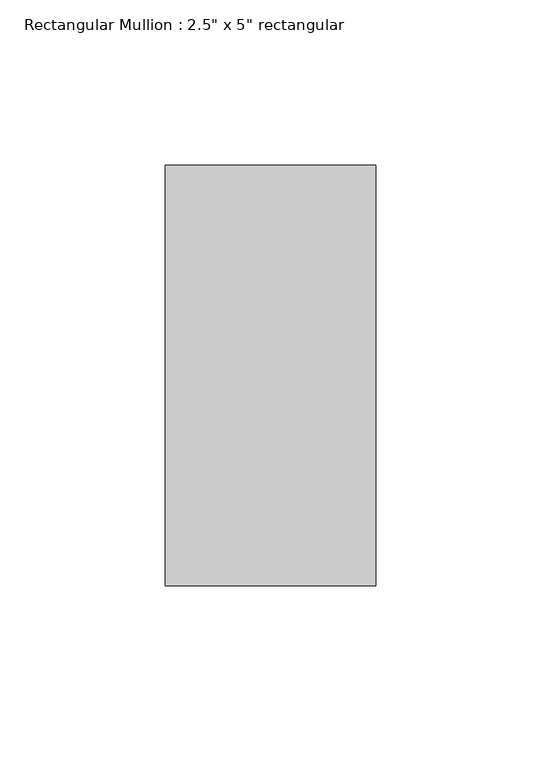
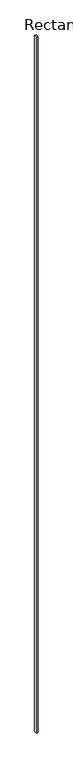
"""IFC4 building model written with IfcOpenShell, lengths in millimetres: member geometry."""

from ifc_helpers import new_model, si_unit, frame, origin, place, context, project, spatial, polyline, outline, extrude, source, transform, mapped, element, save


def member_94459976(model_context):
    return source(origin(), model_context, "Body", "SweptSolid", [
        extrude(outline(polyline([(0.0, 63.5), (0.0, -63.5), (-63.5, -63.5), (-63.5, 63.5), (0.0, 63.5)])), frame((0.0, 0.0, -29260.8), z_axis=(0.0, 0.0, 1.0), x_axis=(1.0, 0.0, 0.0)), (0.0, 0.0, 1.0), 29260.8),
    ])


if __name__ == "__main__":
    model = new_model("IFC4")
    model_context = context("Model", 3, world=origin())
    ifc_project = project(units=[si_unit("LENGTHUNIT", "METRE", prefix="MILLI")], contexts=[model_context])
    site = spatial("IfcSite", under=ifc_project)
    building = spatial("IfcBuilding", under=site)
    placement = place(None, origin())
    member_shape = member_94459976(model_context)
    element("IfcMember", 1, ObjectType="Rectangular Mullion : 2.5\" x 5\" rectangular", at=placement, inside=building, context=model_context, shape_type="MappedRepresentation", body=[
        mapped(member_shape, transform((0.0, 0.0, 0.0), x_axis=(1.0, 0.0, 0.0), y_axis=(0.0, 1.0, 0.0), z_axis=(0.0, 0.0, 1.0))),
    ])
    save(model, "model.ifc")

# Revit data of these elements
# Type "Rectangular Mullion : 2.5\" x 5\" rectangular"
#   built-in parameter 1007304 = 0.416667 (stored number, unit not read)
#   built-in parameter 1007301 = 0.104167 (stored number, unit not read)
#   built-in parameter 1007300 = 0.104167 (stored number, unit not read)
# Element 1 (IfcMember, "Rectangular Mullion : 2.5\" x 5\" rectangular")
#   Materials on its faces: "Aluminum"
# Materials
#   "Aluminum": class "Metal", colour RGB 247 247 247, transparency 0, Description = "Aluminum 6061", Cost = 0
